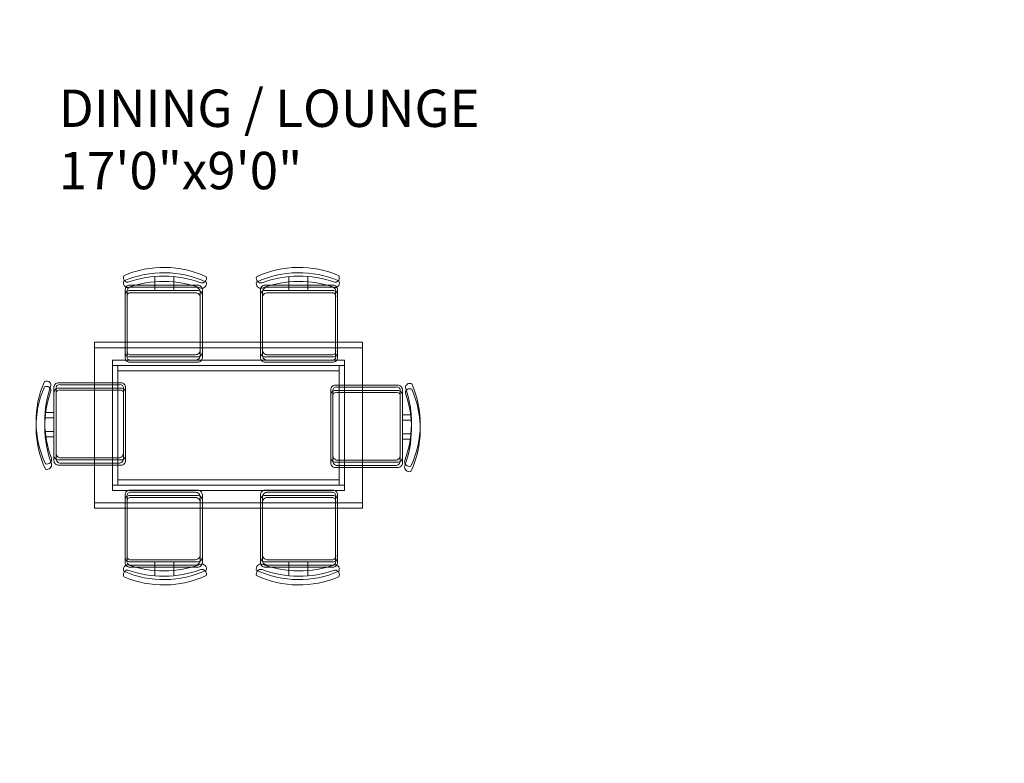
# Model space of a CAD drawing. Units: inches. Extents: x 963 to 2075, y 289 to 2657.
# Tile 14 of 98: x 1179 to 1310, y 1718 to 1818. Entities that reach past the tile are written whole.
import ezdxf

# ---------------------------------------------------------------- set-up
doc = ezdxf.new("R2010")
doc.units = ezdxf.units.IN
for name, color, linetype, lineweight in [('A-AREA-IDEN', 7, 'Continuous', 18), ('A-FURN', 8, 'Continuous', 18), ('A-WALL-PATT', 8, 'Continuous', 13)]:
    doc.layers.add(name, color=color, linetype=linetype, lineweight=lineweight)
doc.styles.get("Standard").update_dxf_attribs({"font": 'arial.ttf'})

msp = doc.modelspace()

# ---------------------------------------------------------------- hatches: boundary and pattern name
at = {"layer": 'A-WALL-PATT'}
h = msp.add_hatch(dxfattribs=at)
h.set_pattern_fill('ANSI32', color=256)
h.paths.add_polyline_path([(1296.92, 2558.32), (1203.92, 2558.32), (1203.92, 2493.82), (1191.53, 2493.82), (1191.53, 2489.32), (1211.06, 2489.32), (1211.06, 2492.02), (1211.06, 2493.82), (1208.42, 2493.82), (1208.42, 2553.82), (1292.42, 2553.82), (1292.42, 2538.86), (1296.92, 2538.86)])
h.paths.add_polyline_path([(1442.42, 2558.32), (1349.42, 2558.32), (1349.42, 2538.94), (1353.92, 2538.94), (1353.92, 2553.82), (1437.92, 2553.82), (1437.92, 2493.82), (1434.54, 2493.82), (1434.54, 2489.32), (1448.31, 2489.32), (1448.31, 2491.57), (1448.31, 2493.82), (1442.42, 2493.82)])
h.paths.add_polyline_path([(1415.55, 2491.57), (1415.55, 2493.82), (1340.94, 2493.82), (1340.94, 2489.32), (1371.92, 2489.32), (1371.92, 2378.32), (1367.6, 2378.32), (1367.6, 2373.82), (1371.92, 2373.82), (1371.92, 2355.19), (1376.42, 2355.19), (1376.42, 2489.32), (1415.55, 2489.32)])
h.paths.add_polyline_path([(1304.94, 2491.57), (1304.94, 2493.82), (1296.92, 2493.82), (1296.92, 2514.86), (1292.42, 2514.86), (1292.42, 2493.82), (1232.81, 2493.82), (1232.81, 2489.32), (1256.42, 2489.32), (1256.42, 2327.32), (1253.71, 2327.32), (1253.71, 2322.82), (1328.42, 2322.82), (1328.42, 2331.15), (1323.92, 2331.15), (1323.92, 2327.32), (1260.92, 2327.32), (1260.92, 2373.82), (1323.92, 2373.82), (1323.92, 2357.81), (1328.42, 2357.81), (1328.42, 2373.82), (1346.01, 2373.82), (1346.01, 2376.07), (1346.01, 2378.32), (1260.92, 2378.32), (1260.92, 2489.32), (1304.94, 2489.32)])
h.paths.add_polyline_path([(1226.65, 2327.32), (1124.42, 2327.32), (1124.42, 2347.45), (1119.92, 2347.45), (1119.92, 2322.82), (1163.42, 2322.82), (1163.42, 2305.43), (1165.67, 2305.43), (1167.92, 2305.43), (1167.92, 2322.82), (1226.65, 2322.82), (1226.65, 2325.07)])
h.paths.add_polyline_path([(1095.92, 2489.32), (1124.42, 2489.32), (1131.53, 2489.32), (1131.53, 2491.57), (1131.53, 2493.82), (1119.92, 2493.82), (1091.42, 2493.82), (1091.42, 2417.32), (1095.92, 2417.32), (1119.92, 2417.32), (1119.92, 2407.45), (1124.42, 2407.45), (1124.42, 2421.82), (1095.92, 2421.82)])
h.paths.add_polyline_path([(1512.92, 2558.32), (1508.42, 2558.32), (1508.42, 2493.82), (1503.4, 2493.82), (1503.4, 2489.32), (1508.42, 2489.32), (1508.42, 2327.32), (1376.42, 2327.32), (1376.42, 2330.27), (1371.92, 2330.27), (1371.92, 2298.74), (1376.42, 2298.74), (1376.42, 2322.82), (1508.42, 2322.82), (1508.42, 2165.32), (1504.26, 2165.32), (1504.26, 2160.82), (1508.42, 2160.82), (1508.42, 2108.32), (1512.92, 2108.32), (1512.92, 2160.82), (1516.18, 2160.82), (1516.18, 2163.07), (1516.18, 2165.32), (1512.92, 2165.32), (1512.92, 2322.82), (1644.92, 2322.82), (1644.92, 2298.74), (1649.42, 2298.74), (1649.42, 2322.82), (1649.42, 2330.94), (1647.17, 2330.94), (1644.92, 2330.94), (1644.92, 2327.32), (1512.92, 2327.32), (1512.92, 2489.32), (1516.76, 2489.32), (1516.76, 2491.57), (1516.76, 2493.82), (1512.92, 2493.82)])
h.paths.add_polyline_path([(1671.92, 2558.32), (1578.92, 2558.32), (1578.92, 2493.82), (1573.53, 2493.82), (1573.53, 2489.32), (1586.54, 2489.32), (1586.54, 2491.57), (1586.54, 2493.82), (1583.42, 2493.82), (1583.42, 2553.82), (1667.42, 2553.82), (1667.42, 2541.11), (1671.92, 2541.11)])
h.paths.add_polyline_path([(1681.26, 2493.82), (1671.92, 2493.82), (1671.92, 2517.11), (1667.42, 2517.11), (1667.42, 2493.82), (1610.22, 2493.82), (1610.22, 2489.32), (1644.92, 2489.32), (1644.92, 2357.87), (1649.42, 2357.87), (1649.42, 2373.82), (1652.2, 2373.82), (1652.2, 2375.83), (1652.2, 2378.32), (1649.42, 2378.32), (1649.42, 2489.32), (1681.26, 2489.32), (1681.26, 2491.57)])
h.paths.add_polyline_path([(1821.92, 2558.32), (1728.92, 2558.32), (1728.92, 2541), (1733.42, 2541), (1733.42, 2553.82), (1817.42, 2553.82), (1817.42, 2493.82), (1813.51, 2493.82), (1813.51, 2489.32), (1830.08, 2489.32), (1830.08, 2491.57), (1830.08, 2493.82), (1821.92, 2493.82)])
h.paths.add_polyline_path([(1794.24, 2493.82), (1717.26, 2493.82), (1717.26, 2489.32), (1760.42, 2489.32), (1760.42, 2378.32), (1674.4, 2378.32), (1674.4, 2373.82), (1692.92, 2373.82), (1692.92, 2356.95), (1697.42, 2356.95), (1697.42, 2373.82), (1760.42, 2373.82), (1760.42, 2327.32), (1697.42, 2327.32), (1697.42, 2333.34), (1692.92, 2333.34), (1692.92, 2322.82), (1768.04, 2322.82), (1768.04, 2325.07), (1768.04, 2327.32), (1764.92, 2327.32), (1764.92, 2489.32), (1794.24, 2489.32)])
h.paths.add_polyline_path([(1733.42, 2517), (1728.92, 2517), (1728.92, 2493.82), (1733.42, 2493.82)], flags=17)
h.paths.add_polyline_path([(1929.92, 2493.82), (1890.08, 2493.82), (1890.08, 2489.32), (1896.92, 2489.32), (1925.42, 2489.32), (1925.42, 2421.82), (1896.92, 2421.82), (1896.92, 2408.32), (1901.42, 2408.32), (1901.42, 2417.32), (1925.42, 2417.32), (1929.92, 2417.32)])
h.paths.add_polyline_path([(1901.42, 2348.32), (1896.92, 2348.32), (1896.92, 2327.32), (1800.42, 2327.32), (1800.42, 2322.82), (1853.42, 2322.82), (1853.42, 2309.45), (1857.92, 2309.45), (1857.92, 2322.82), (1901.42, 2322.82)])
h.paths.add_polyline_path([(1857.92, 2249.45), (1853.42, 2249.45), (1853.42, 2214.82), (1686.31, 2214.82), (1686.31, 2210.32), (1853.42, 2210.32), (1853.42, 2202.13), (1857.92, 2202.13), (1857.92, 2210.32)])
h.paths.add_polyline_path([(1857.92, 2142.13), (1853.42, 2142.13), (1853.42, 2115.42), (1841.42, 2115.42), (1841.42, 2088.53), (1841.42, 2046.95), (1845.92, 2046.95), (1845.92, 2110.92), (1905.92, 2110.92), (1905.92, 2092.52), (1910.42, 2092.52), (1910.42, 2115.42), (1857.92, 2115.42)])
h.paths.add_polyline_path([(1532.44, 1482.34), (1573.46, 1482.34), (1573.46, 1501), (1532.44, 1501)], flags=9)
h.paths.add_polyline_path([(1438.66, 1486.3), (1479.68, 1486.3), (1479.68, 1504.96), (1438.66, 1504.96)], flags=9)
h.paths.add_polyline_path([(1411.22, 1365.31), (1659.14, 1365.31), (1659.14, 1402.4), (1411.22, 1402.4)], flags=9)
h.paths.add_polyline_path([(1185.67, 2296.3), (1248.16, 2296.3), (1248.16, 2314.95), (1185.67, 2314.95)], flags=9)
h.paths.add_polyline_path([(1177.31, 2187.35), (1216.15, 2187.35), (1216.15, 2206.01), (1177.31, 2206.01)], flags=9)
h.paths.add_polyline_path([(1295.1, 1602.08), (1328.26, 1602.08), (1328.26, 1620.74), (1295.1, 1620.74)], flags=9)
h.paths.add_polyline_path([(1525.13, 2005.99), (1558.39, 2005.99), (1558.39, 2024.65), (1525.13, 2024.65)], flags=9)
h.paths.add_polyline_path([(1459.61, 1977.13), (1472.19, 1977.13), (1472.19, 1987.43), (1459.61, 1987.43)], flags=9)
h.paths.add_polyline_path([(1467.81, 2053.68), (1480.02, 2053.68), (1480.02, 2063.98), (1467.81, 2063.98)], flags=9)
h.paths.add_polyline_path([(1555.18, 2119.02), (1584.56, 2119.02), (1584.56, 2137.68), (1555.18, 2137.68)], flags=25)
h.paths.add_polyline_path([(1405.39, 2115.29), (1444.48, 2115.29), (1444.48, 2133.95), (1405.39, 2133.95)], flags=25)
h.paths.add_polyline_path([(1698.48, 2004.26), (1727.69, 2004.26), (1727.69, 2022.92), (1698.48, 2022.92)], flags=9)
h.paths.add_polyline_path([(1612.16, 1972.86), (1629.02, 1972.86), (1629.02, 1983.16), (1612.16, 1983.16)], flags=9)
h.paths.add_polyline_path([(1608.29, 2060.04), (1625.15, 2060.04), (1625.15, 2070.34), (1608.29, 2070.34)], flags=9)
h.paths.add_polyline_path([(1527.95, 1684.4), (1566.79, 1684.4), (1566.79, 1703.06), (1527.95, 1703.06)], flags=9)
h.paths.add_polyline_path([(1422.79, 1683.59), (1461.63, 1683.59), (1461.63, 1702.25), (1422.79, 1702.25)], flags=9)
h.paths.add_polyline_path([(1531.26, 1732.46), (1574.01, 1732.46), (1574.01, 1751.12), (1531.26, 1751.12)], flags=9)
h.paths.add_polyline_path([(1402.87, 1732.85), (1439.8, 1732.85), (1439.8, 1751.5), (1402.87, 1751.5)], flags=9)
h.paths.add_polyline_path([(1243.12, 1923.13), (1281.96, 1923.13), (1281.96, 1941.79), (1243.12, 1941.79)], flags=9)
h.paths.add_polyline_path([(1181.75, 1792.27), (1244.24, 1792.27), (1244.24, 1810.93), (1181.75, 1810.93)], flags=9)
h.paths.add_polyline_path([(1265.82, 1670.3), (1316.07, 1670.3), (1316.07, 1688.96), (1265.82, 1688.96)], flags=9)
h.paths.add_polyline_path([(1140.26, 1676.05), (1179.1, 1676.05), (1179.1, 1694.71), (1140.26, 1694.71)], flags=9)
h.paths.add_polyline_path([(1107.49, 1490.89), (1143.37, 1490.89), (1143.37, 1509.55), (1107.49, 1509.55)], flags=9)
h.paths.add_polyline_path([(1217.58, 1483.9), (1246.74, 1483.9), (1246.74, 1502.56), (1217.58, 1502.56)], flags=9)
h.paths.add_polyline_path([(1389.21, 1486.92), (1418.37, 1486.92), (1418.37, 1505.58), (1389.21, 1505.58)], flags=9)
h.paths.add_polyline_path([(1672.21, 1602.08), (1705.37, 1602.08), (1705.37, 1620.74), (1672.21, 1620.74)], flags=9)
h.paths.add_polyline_path([(1752.08, 1522.64), (1781.24, 1522.64), (1781.24, 1541.3), (1752.08, 1541.3)], flags=9)
h.paths.add_polyline_path([(1848.27, 1491.26), (1884.16, 1491.26), (1884.16, 1509.92), (1848.27, 1509.92)], flags=9)
h.paths.add_polyline_path([(1822.47, 1685.62), (1861.31, 1685.62), (1861.31, 1704.28), (1822.47, 1704.28)], flags=9)
h.paths.add_polyline_path([(1713.19, 1672.23), (1763.44, 1672.23), (1763.44, 1690.89), (1713.19, 1690.89)], flags=9)
h.paths.add_polyline_path([(1736.62, 1790.58), (1799.11, 1790.58), (1799.11, 1809.24), (1736.62, 1809.24)], flags=9)
h.paths.add_polyline_path([(1691.49, 1916.36), (1730.33, 1916.36), (1730.33, 1935.01), (1691.49, 1935.01)], flags=9)
h.paths.add_polyline_path([(1764.87, 1973.92), (1794.31, 1973.92), (1794.31, 1992.58), (1764.87, 1992.58)], flags=9)
h.paths.add_polyline_path([(1767.85, 2034.02), (1797.29, 2034.02), (1797.29, 2052.67), (1767.85, 2052.67)], flags=9)
h.paths.add_polyline_path([(1851.59, 2060.33), (1880.75, 2060.33), (1880.75, 2078.99), (1851.59, 2078.99)], flags=25)
h.paths.add_polyline_path([(1688.49, 2086.87), (1727.33, 2086.87), (1727.33, 2105.53), (1688.49, 2105.53)], flags=9)
h.paths.add_polyline_path([(1537.74, 2293.58), (1580.49, 2293.58), (1580.49, 2312.24), (1537.74, 2312.24)], flags=25)
h.paths.add_polyline_path([(1425.59, 2296.11), (1468.34, 2296.11), (1468.34, 2314.77), (1425.59, 2314.77)], flags=25)
h.paths.add_polyline_path([(1278.52, 2004.18), (1307.72, 2004.18), (1307.72, 2022.84), (1278.52, 2022.84)], flags=9)
h.paths.add_polyline_path([(1193.28, 1973.63), (1222.72, 1973.63), (1222.72, 1992.29), (1193.28, 1992.29)], flags=9)
h.paths.add_polyline_path([(1192.41, 2040.58), (1221.84, 2040.58), (1221.84, 2059.23), (1192.41, 2059.23)], flags=9)
h.paths.add_polyline_path([(1130.6, 1951.39), (1159.76, 1951.39), (1159.76, 1970.05), (1130.6, 1970.05)], flags=9)
h.paths.add_polyline_path([(1132.83, 2052.49), (1161.98, 2052.49), (1161.98, 2071.15), (1132.83, 2071.15)], flags=9)
h.paths.add_polyline_path([(1265.13, 2334.62), (1315.38, 2334.62), (1315.38, 2353.28), (1265.13, 2353.28)], flags=25)
h.paths.add_polyline_path([(1136.74, 2330.79), (1175.58, 2330.79), (1175.58, 2349.44), (1136.74, 2349.44)], flags=9)
h.paths.add_polyline_path([(1287.42, 2417.2), (1320.58, 2417.2), (1320.58, 2435.86), (1287.42, 2435.86)], flags=25)
h.paths.add_polyline_path([(1430.99, 2329.16), (1469.83, 2329.16), (1469.83, 2347.82), (1430.99, 2347.82)], flags=25)
h.paths.add_polyline_path([(1525.42, 2329.21), (1564.26, 2329.21), (1564.26, 2347.87), (1525.42, 2347.87)], flags=25)
h.paths.add_polyline_path([(1684.52, 2382.8), (1717.68, 2382.8), (1717.68, 2401.46), (1684.52, 2401.46)], flags=25)
h.paths.add_polyline_path([(1704.81, 2340.29), (1755.05, 2340.29), (1755.05, 2358.95), (1704.81, 2358.95)], flags=25)
h.paths.add_polyline_path([(1694.11, 2287.76), (1756.6, 2287.76), (1756.6, 2306.41), (1694.11, 2306.41)], flags=9)
h.paths.add_polyline_path([(1815.78, 2329.86), (1854.62, 2329.86), (1854.62, 2348.52), (1815.78, 2348.52)], flags=9)
h.paths.add_polyline_path([(1842.87, 2514.26), (1878.76, 2514.26), (1878.76, 2532.91), (1842.87, 2532.91)], flags=9)
h.paths.add_polyline_path([(1769.51, 2531.45), (1798.67, 2531.45), (1798.67, 2550.1), (1769.51, 2550.1)], flags=25)
h.paths.add_polyline_path([(1594.77, 2518.47), (1623.93, 2518.47), (1623.93, 2537.13), (1594.77, 2537.13)], flags=25)
h.paths.add_polyline_path([(1520.72, 2516.18), (1556.61, 2516.18), (1556.61, 2534.84), (1520.72, 2534.84)], flags=25)
h.paths.add_polyline_path([(1464.46, 2516.69), (1500.34, 2516.69), (1500.34, 2535.35), (1464.46, 2535.35)], flags=25)
h.paths.add_polyline_path([(1365.7, 2528.97), (1394.85, 2528.97), (1394.85, 2547.63), (1365.7, 2547.63)], flags=25)
h.paths.add_polyline_path([(1222.84, 2516.23), (1252, 2516.23), (1252, 2534.89), (1222.84, 2534.89)], flags=25)
h.paths.add_polyline_path([(1104.55, 2509.6), (1140.43, 2509.6), (1140.43, 2528.26), (1104.55, 2528.26)], flags=9)
h = msp.add_hatch(dxfattribs=at)
h.set_pattern_fill('ANSI32', color=256)
h.paths.add_polyline_path([(1335.97, 2212.57), (1335.97, 2214.82), (1167.92, 2214.82), (1167.92, 2245.43), (1163.42, 2245.43), (1163.42, 2210.32), (1163.42, 2194.81), (1167.92, 2194.81), (1167.92, 2210.32), (1335.97, 2210.32)])
h.paths.add_polyline_path([(1532.44, 1482.34), (1573.46, 1482.34), (1573.46, 1501), (1532.44, 1501)], flags=9)
h.paths.add_polyline_path([(1438.66, 1486.3), (1479.68, 1486.3), (1479.68, 1504.96), (1438.66, 1504.96)], flags=9)
h.paths.add_polyline_path([(1411.22, 1365.31), (1659.14, 1365.31), (1659.14, 1402.4), (1411.22, 1402.4)], flags=9)
h.paths.add_polyline_path([(1185.67, 2296.3), (1248.16, 2296.3), (1248.16, 2314.95), (1185.67, 2314.95)], flags=9)
h.paths.add_polyline_path([(1177.31, 2187.35), (1216.15, 2187.35), (1216.15, 2206.01), (1177.31, 2206.01)], flags=9)
h.paths.add_polyline_path([(1295.1, 1602.08), (1328.26, 1602.08), (1328.26, 1620.74), (1295.1, 1620.74)], flags=9)
h.paths.add_polyline_path([(1525.13, 2005.99), (1558.39, 2005.99), (1558.39, 2024.65), (1525.13, 2024.65)], flags=9)
h.paths.add_polyline_path([(1459.61, 1977.13), (1472.19, 1977.13), (1472.19, 1987.43), (1459.61, 1987.43)], flags=9)
h.paths.add_polyline_path([(1467.81, 2053.68), (1480.02, 2053.68), (1480.02, 2063.98), (1467.81, 2063.98)], flags=9)
h.paths.add_polyline_path([(1555.18, 2119.02), (1584.56, 2119.02), (1584.56, 2137.68), (1555.18, 2137.68)], flags=9)
h.paths.add_polyline_path([(1405.39, 2115.29), (1444.48, 2115.29), (1444.48, 2133.95), (1405.39, 2133.95)], flags=9)
h.paths.add_polyline_path([(1698.48, 2004.26), (1727.69, 2004.26), (1727.69, 2022.92), (1698.48, 2022.92)], flags=9)
h.paths.add_polyline_path([(1612.16, 1972.86), (1629.02, 1972.86), (1629.02, 1983.16), (1612.16, 1983.16)], flags=9)
h.paths.add_polyline_path([(1608.29, 2060.04), (1625.15, 2060.04), (1625.15, 2070.34), (1608.29, 2070.34)], flags=9)
h.paths.add_polyline_path([(1527.95, 1684.4), (1566.79, 1684.4), (1566.79, 1703.06), (1527.95, 1703.06)], flags=9)
h.paths.add_polyline_path([(1422.79, 1683.59), (1461.63, 1683.59), (1461.63, 1702.25), (1422.79, 1702.25)], flags=9)
h.paths.add_polyline_path([(1531.26, 1732.46), (1574.01, 1732.46), (1574.01, 1751.12), (1531.26, 1751.12)], flags=9)
h.paths.add_polyline_path([(1402.87, 1732.85), (1439.8, 1732.85), (1439.8, 1751.5), (1402.87, 1751.5)], flags=9)
h.paths.add_polyline_path([(1243.12, 1923.13), (1281.96, 1923.13), (1281.96, 1941.79), (1243.12, 1941.79)], flags=9)
h.paths.add_polyline_path([(1181.75, 1792.27), (1244.24, 1792.27), (1244.24, 1810.93), (1181.75, 1810.93)], flags=9)
h.paths.add_polyline_path([(1265.82, 1670.3), (1316.07, 1670.3), (1316.07, 1688.96), (1265.82, 1688.96)], flags=9)
h.paths.add_polyline_path([(1140.26, 1676.05), (1179.1, 1676.05), (1179.1, 1694.71), (1140.26, 1694.71)], flags=9)
h.paths.add_polyline_path([(1107.49, 1490.89), (1143.37, 1490.89), (1143.37, 1509.55), (1107.49, 1509.55)], flags=9)
h.paths.add_polyline_path([(1217.58, 1483.9), (1246.74, 1483.9), (1246.74, 1502.56), (1217.58, 1502.56)], flags=9)
h.paths.add_polyline_path([(1389.21, 1486.92), (1418.37, 1486.92), (1418.37, 1505.58), (1389.21, 1505.58)], flags=9)
h.paths.add_polyline_path([(1672.21, 1602.08), (1705.37, 1602.08), (1705.37, 1620.74), (1672.21, 1620.74)], flags=9)
h.paths.add_polyline_path([(1752.08, 1522.64), (1781.24, 1522.64), (1781.24, 1541.3), (1752.08, 1541.3)], flags=9)
h.paths.add_polyline_path([(1848.27, 1491.26), (1884.16, 1491.26), (1884.16, 1509.92), (1848.27, 1509.92)], flags=9)
h.paths.add_polyline_path([(1822.47, 1685.62), (1861.31, 1685.62), (1861.31, 1704.28), (1822.47, 1704.28)], flags=9)
h.paths.add_polyline_path([(1713.19, 1672.23), (1763.44, 1672.23), (1763.44, 1690.89), (1713.19, 1690.89)], flags=9)
h.paths.add_polyline_path([(1736.62, 1790.58), (1799.11, 1790.58), (1799.11, 1809.24), (1736.62, 1809.24)], flags=9)
h.paths.add_polyline_path([(1691.49, 1916.36), (1730.33, 1916.36), (1730.33, 1935.01), (1691.49, 1935.01)], flags=9)
h.paths.add_polyline_path([(1764.87, 1973.92), (1794.31, 1973.92), (1794.31, 1992.58), (1764.87, 1992.58)], flags=9)
h.paths.add_polyline_path([(1767.85, 2034.02), (1797.29, 2034.02), (1797.29, 2052.67), (1767.85, 2052.67)], flags=9)
h.paths.add_polyline_path([(1851.59, 2060.33), (1880.75, 2060.33), (1880.75, 2078.99), (1851.59, 2078.99)], flags=9)
h.paths.add_polyline_path([(1688.49, 2086.87), (1727.33, 2086.87), (1727.33, 2105.53), (1688.49, 2105.53)], flags=9)
h.paths.add_polyline_path([(1537.74, 2293.58), (1580.49, 2293.58), (1580.49, 2312.24), (1537.74, 2312.24)], flags=9)
h.paths.add_polyline_path([(1425.59, 2296.11), (1468.34, 2296.11), (1468.34, 2314.77), (1425.59, 2314.77)], flags=9)
h.paths.add_polyline_path([(1278.52, 2004.18), (1307.72, 2004.18), (1307.72, 2022.84), (1278.52, 2022.84)], flags=9)
h.paths.add_polyline_path([(1193.28, 1973.63), (1222.72, 1973.63), (1222.72, 1992.29), (1193.28, 1992.29)], flags=9)
h.paths.add_polyline_path([(1192.41, 2040.58), (1221.84, 2040.58), (1221.84, 2059.23), (1192.41, 2059.23)], flags=9)
h.paths.add_polyline_path([(1130.6, 1951.39), (1159.76, 1951.39), (1159.76, 1970.05), (1130.6, 1970.05)], flags=9)
h.paths.add_polyline_path([(1132.83, 2052.49), (1161.98, 2052.49), (1161.98, 2071.15), (1132.83, 2071.15)], flags=9)
h.paths.add_polyline_path([(1265.13, 2334.62), (1315.38, 2334.62), (1315.38, 2353.28), (1265.13, 2353.28)], flags=9)
h.paths.add_polyline_path([(1136.74, 2330.79), (1175.58, 2330.79), (1175.58, 2349.44), (1136.74, 2349.44)], flags=9)
h.paths.add_polyline_path([(1287.42, 2417.2), (1320.58, 2417.2), (1320.58, 2435.86), (1287.42, 2435.86)], flags=9)
h.paths.add_polyline_path([(1430.99, 2329.16), (1469.83, 2329.16), (1469.83, 2347.82), (1430.99, 2347.82)], flags=9)
h.paths.add_polyline_path([(1525.42, 2329.21), (1564.26, 2329.21), (1564.26, 2347.87), (1525.42, 2347.87)], flags=9)
h.paths.add_polyline_path([(1684.52, 2382.8), (1717.68, 2382.8), (1717.68, 2401.46), (1684.52, 2401.46)], flags=9)
h.paths.add_polyline_path([(1704.81, 2340.29), (1755.05, 2340.29), (1755.05, 2358.95), (1704.81, 2358.95)], flags=9)
h.paths.add_polyline_path([(1694.11, 2287.76), (1756.6, 2287.76), (1756.6, 2306.41), (1694.11, 2306.41)], flags=9)
h.paths.add_polyline_path([(1815.78, 2329.86), (1854.62, 2329.86), (1854.62, 2348.52), (1815.78, 2348.52)], flags=9)
h.paths.add_polyline_path([(1842.87, 2514.26), (1878.76, 2514.26), (1878.76, 2532.91), (1842.87, 2532.91)], flags=9)
h.paths.add_polyline_path([(1769.51, 2531.45), (1798.67, 2531.45), (1798.67, 2550.1), (1769.51, 2550.1)], flags=9)
h.paths.add_polyline_path([(1594.77, 2518.47), (1623.93, 2518.47), (1623.93, 2537.13), (1594.77, 2537.13)], flags=9)
h.paths.add_polyline_path([(1520.72, 2516.18), (1556.61, 2516.18), (1556.61, 2534.84), (1520.72, 2534.84)], flags=9)
h.paths.add_polyline_path([(1464.46, 2516.69), (1500.34, 2516.69), (1500.34, 2535.35), (1464.46, 2535.35)], flags=9)
h.paths.add_polyline_path([(1365.7, 2528.97), (1394.85, 2528.97), (1394.85, 2547.63), (1365.7, 2547.63)], flags=9)
h.paths.add_polyline_path([(1222.84, 2516.23), (1252, 2516.23), (1252, 2534.89), (1222.84, 2534.89)], flags=9)
h.paths.add_polyline_path([(1104.55, 2509.6), (1140.43, 2509.6), (1140.43, 2528.26), (1104.55, 2528.26)], flags=9)

# ---------------------------------------------------------------- linework, layer by layer
at = {"layer": 'A-FURN'}
for points in [[(1193, 1782.66, -0.175809), (1202.76, 1782.58, 0.578392), (1203.5, 1783.4, 0.214524), (1192.49, 1783.54, 0.552014), (1193, 1782.66, -0.065079)], [(1193, 1782.66, -0.175809), (1202.76, 1782.58, 0.578392), (1203.5, 1783.4, 0.214524), (1192.49, 1783.54, 0.552014), (1193, 1782.66, -0.065079)], [(1193, 1781.94, -0.175809), (1202.76, 1781.87, 0.578392), (1203.5, 1782.68, 0.214524), (1192.49, 1782.83, 0.552014), (1193, 1781.94, -0.065079)], [(1193, 1781.94, -0.175809), (1202.76, 1781.87, 0.578392), (1203.5, 1782.68, 0.214524), (1192.49, 1782.83, 0.552014), (1193, 1781.94, -0.065079)], [(1210.97, 1782.58, -0.578392), (1210.23, 1783.4, -0.214524), (1221.24, 1783.54, -0.552014), (1220.72, 1782.66, 0.175809), (1210.97, 1782.58)], [(1210.97, 1782.58, -0.578392), (1210.23, 1783.4, -0.214524), (1221.24, 1783.54, -0.552014), (1220.72, 1782.66, 0.175809), (1210.97, 1782.58)], [(1210.97, 1781.87, -0.578392), (1210.23, 1782.68, -0.214524), (1221.24, 1782.83, -0.552014), (1220.72, 1781.94, 0.175809), (1210.97, 1781.87)], [(1210.97, 1781.87, -0.578392), (1210.23, 1782.68, -0.214524), (1221.24, 1782.83, -0.552014), (1220.72, 1781.94, 0.175809), (1210.97, 1781.87)], [(1199.16, 1782.27), (1199.16, 1783.41, -0.064759)], [(1199.16, 1782.27), (1199.16, 1783.41, -0.064759)], [(1199.16, 1781.55), (1199.16, 1782.69, -0.064759)], [(1199.16, 1781.55), (1199.16, 1782.69, -0.064759)], [(1214.56, 1782.27), (1214.56, 1783.41, 0.064759)], [(1214.56, 1782.27), (1214.56, 1783.41, 0.064759)], [(1214.56, 1781.55), (1214.56, 1782.69, 0.064759)], [(1214.56, 1781.55), (1214.56, 1782.69, 0.064759)], [(1202.34, 1782.27), (1193.29, 1782.27, 0.414214), (1192.65, 1781.63), (1192.65, 1773.31, 0.414214), (1193.29, 1772.67), (1202.34, 1772.67, 0.414214), (1202.98, 1773.31), (1202.98, 1781.63, 0.414214), (1202.34, 1782.27)], [(1202.34, 1781.55), (1193.29, 1781.55, 0.414214), (1192.65, 1780.92), (1192.65, 1772.59, 0.414214), (1193.29, 1771.96), (1202.34, 1771.96, 0.414214), (1202.98, 1772.59), (1202.98, 1780.92, 0.414214), (1202.34, 1781.55)], [(1202.34, 1782.27), (1193.29, 1782.27, 0.414214), (1192.65, 1781.63), (1192.65, 1773.31, 0.414214), (1193.29, 1772.67), (1202.34, 1772.67, 0.414214), (1202.98, 1773.31), (1202.98, 1781.63, 0.414214), (1202.34, 1782.27)], [(1202.34, 1781.55), (1193.29, 1781.55, 0.414214), (1192.65, 1780.92), (1192.65, 1772.59, 0.414214), (1193.29, 1771.96), (1202.34, 1771.96, 0.414214), (1202.98, 1772.59), (1202.98, 1780.92, 0.414214), (1202.34, 1781.55)], [(1220.44, 1782.27, -0.414214), (1221.07, 1781.63), (1221.07, 1773.31, -0.414214), (1220.44, 1772.67), (1211.38, 1772.67, -0.414214), (1210.75, 1773.31), (1210.75, 1781.63, -0.414214), (1211.38, 1782.27), (1220.44, 1782.27)], [(1220.44, 1782.27, -0.414214), (1221.07, 1781.63), (1221.07, 1773.31, -0.414214), (1220.44, 1772.67), (1211.38, 1772.67, -0.414214), (1210.75, 1773.31), (1210.75, 1781.63, -0.414214), (1211.38, 1782.27), (1220.44, 1782.27)], [(1220.44, 1781.55, -0.414214), (1221.07, 1780.92), (1221.07, 1772.59, -0.414214), (1220.44, 1771.96), (1211.38, 1771.96, -0.414214), (1210.75, 1772.59), (1210.75, 1780.92, -0.414214), (1211.38, 1781.55), (1220.44, 1781.55)], [(1220.44, 1781.55, -0.414214), (1221.07, 1780.92), (1221.07, 1772.59, -0.414214), (1220.44, 1771.96), (1211.38, 1771.96, -0.414214), (1210.75, 1772.59), (1210.75, 1780.92, -0.414214), (1211.38, 1781.55), (1220.44, 1781.55)], [(1182.8, 1759.1, -0.578392), (1181.99, 1758.36, -0.214524), (1181.84, 1769.37, -0.552014), (1182.73, 1768.86, 0.175809), (1182.8, 1759.1)], [(1182.8, 1759.1, -0.578392), (1181.99, 1758.36, -0.214524), (1181.84, 1769.37, -0.552014), (1182.73, 1768.86, 0.175809), (1182.8, 1759.1)], [(1183.12, 1768.57, -0.414214), (1183.75, 1769.21), (1192.08, 1769.21, -0.414214), (1192.71, 1768.57), (1192.71, 1759.52, -0.414214), (1192.08, 1758.88), (1183.75, 1758.88, -0.414214), (1183.12, 1759.52), (1183.12, 1768.57)], [(1183.12, 1768.57, -0.414214), (1183.75, 1769.21), (1192.08, 1769.21, -0.414214), (1192.71, 1768.57), (1192.71, 1759.52, -0.414214), (1192.08, 1758.88), (1183.75, 1758.88, -0.414214), (1183.12, 1759.52), (1183.12, 1768.57)], [(1182.8, 1758.39, -0.578392), (1181.99, 1757.65, -0.214524), (1181.84, 1768.66, -0.552014), (1182.73, 1768.14, 0.175809), (1182.8, 1758.39)], [(1182.8, 1758.39, -0.578392), (1181.99, 1757.65, -0.214524), (1181.84, 1768.66, -0.552014), (1182.73, 1768.14, 0.175809), (1182.8, 1758.39)], [(1183.12, 1767.86, -0.414214), (1183.75, 1768.49), (1192.08, 1768.49, -0.414214), (1192.71, 1767.86), (1192.71, 1758.8, -0.414214), (1192.08, 1758.17), (1183.75, 1758.17, -0.414214), (1183.12, 1758.8), (1183.12, 1767.86)], [(1183.12, 1767.86, -0.414214), (1183.75, 1768.49), (1192.08, 1768.49, -0.414214), (1192.71, 1767.86), (1192.71, 1758.8, -0.414214), (1192.08, 1758.17), (1183.75, 1758.17, -0.414214), (1183.12, 1758.8), (1183.12, 1767.86)], [(1229.75, 1768.26, 0.414214), (1229.11, 1768.9), (1220.79, 1768.9, 0.414214), (1220.15, 1768.26), (1220.15, 1759.21, 0.414214), (1220.79, 1758.57), (1229.11, 1758.57, 0.414214), (1229.75, 1759.21), (1229.75, 1768.26)], [(1229.75, 1768.26, 0.414214), (1229.11, 1768.9), (1220.79, 1768.9, 0.414214), (1220.15, 1768.26), (1220.15, 1759.21, 0.414214), (1220.79, 1758.57), (1229.11, 1758.57, 0.414214), (1229.75, 1759.21), (1229.75, 1768.26)], [(1229.75, 1767.55, 0.414214), (1229.11, 1768.18), (1220.79, 1768.18, 0.414214), (1220.15, 1767.55), (1220.15, 1758.49, 0.414214), (1220.79, 1757.86), (1229.11, 1757.86, 0.414214), (1229.75, 1758.49), (1229.75, 1767.55)], [(1229.75, 1767.55, 0.414214), (1229.11, 1768.18), (1220.79, 1768.18, 0.414214), (1220.15, 1767.55), (1220.15, 1758.49, 0.414214), (1220.79, 1757.86), (1229.11, 1757.86, 0.414214), (1229.75, 1758.49), (1229.75, 1767.55)], [(1230.14, 1768.55, -0.175809), (1230.06, 1758.79, 0.578392), (1230.88, 1758.05, 0.214524), (1231.02, 1769.06, 0.552014), (1230.14, 1768.55, -0.065079)], [(1230.14, 1768.55, -0.175809), (1230.06, 1758.79, 0.578392), (1230.88, 1758.05, 0.214524), (1231.02, 1769.06, 0.552014), (1230.14, 1768.55, -0.065079)], [(1230.14, 1767.83, -0.175809), (1230.06, 1758.08, 0.578392), (1230.88, 1757.34, 0.214524), (1231.02, 1768.35, 0.552014), (1230.14, 1767.83, -0.065079)], [(1230.14, 1767.83, -0.175809), (1230.06, 1758.08, 0.578392), (1230.88, 1757.34, 0.214524), (1231.02, 1768.35, 0.552014), (1230.14, 1767.83, -0.065079)], [(1183.12, 1762.7), (1181.97, 1762.7, 0.064759)], [(1183.12, 1762.7), (1181.97, 1762.7, 0.064759)], [(1183.12, 1761.98), (1181.97, 1761.98, 0.064759)], [(1183.12, 1761.98), (1181.97, 1761.98, 0.064759)], [(1229.75, 1762.39), (1230.89, 1762.39, -0.064759)], [(1229.75, 1762.39), (1230.89, 1762.39, -0.064759)], [(1229.75, 1761.67), (1230.89, 1761.67, -0.064759)], [(1229.75, 1761.67), (1230.89, 1761.67, -0.064759)], [(1202.34, 1745.25), (1193.29, 1745.25, -0.414214), (1192.65, 1745.89), (1192.65, 1754.21, -0.414214), (1193.29, 1754.85), (1202.34, 1754.85, -0.414214), (1202.98, 1754.21), (1202.98, 1745.89, -0.414214), (1202.34, 1745.25)], [(1202.34, 1745.25), (1193.29, 1745.25, -0.414214), (1192.65, 1745.89), (1192.65, 1754.21, -0.414214), (1193.29, 1754.85), (1202.34, 1754.85, -0.414214), (1202.98, 1754.21), (1202.98, 1745.89, -0.414214), (1202.34, 1745.25)], [(1220.44, 1745.25, 0.414214), (1221.07, 1745.89), (1221.07, 1754.21, 0.414214), (1220.44, 1754.85), (1211.38, 1754.85, 0.414214), (1210.75, 1754.21), (1210.75, 1745.89, 0.414214), (1211.38, 1745.25), (1220.44, 1745.25)], [(1220.44, 1745.25, 0.414214), (1221.07, 1745.89), (1221.07, 1754.21, 0.414214), (1220.44, 1754.85), (1211.38, 1754.85, 0.414214), (1210.75, 1754.21), (1210.75, 1745.89, 0.414214), (1211.38, 1745.25), (1220.44, 1745.25)], [(1202.34, 1744.54), (1193.29, 1744.54, -0.414214), (1192.65, 1745.17), (1192.65, 1753.5, -0.414214), (1193.29, 1754.13), (1202.34, 1754.13, -0.414214), (1202.98, 1753.5), (1202.98, 1745.17, -0.414214), (1202.34, 1744.54)], [(1202.34, 1744.54), (1193.29, 1744.54, -0.414214), (1192.65, 1745.17), (1192.65, 1753.5, -0.414214), (1193.29, 1754.13), (1202.34, 1754.13, -0.414214), (1202.98, 1753.5), (1202.98, 1745.17, -0.414214), (1202.34, 1744.54)], [(1220.44, 1744.54, 0.414214), (1221.07, 1745.17), (1221.07, 1753.5, 0.414214), (1220.44, 1754.13), (1211.38, 1754.13, 0.414214), (1210.75, 1753.5), (1210.75, 1745.17, 0.414214), (1211.38, 1744.54), (1220.44, 1744.54)], [(1220.44, 1744.54, 0.414214), (1221.07, 1745.17), (1221.07, 1753.5, 0.414214), (1220.44, 1754.13), (1211.38, 1754.13, 0.414214), (1210.75, 1753.5), (1210.75, 1745.17, 0.414214), (1211.38, 1744.54), (1220.44, 1744.54)], [(1202.76, 1744.94, -0.578392), (1203.5, 1744.12, -0.214524), (1192.49, 1743.98, -0.552014), (1193, 1744.86, 0.175809), (1202.76, 1744.94)], [(1202.76, 1744.94, -0.578392), (1203.5, 1744.12, -0.214524), (1192.49, 1743.98, -0.552014), (1193, 1744.86, 0.175809), (1202.76, 1744.94)], [(1202.76, 1744.22, -0.578392), (1203.5, 1743.41, -0.214524), (1192.49, 1743.26, -0.552014), (1193, 1744.15, 0.175809), (1202.76, 1744.22)], [(1202.76, 1744.22, -0.578392), (1203.5, 1743.41, -0.214524), (1192.49, 1743.26, -0.552014), (1193, 1744.15, 0.175809), (1202.76, 1744.22)], [(1199.16, 1745.25), (1199.16, 1744.11, 0.064759)], [(1199.16, 1745.25), (1199.16, 1744.11, 0.064759)], [(1199.16, 1744.54), (1199.16, 1743.39, 0.064759)], [(1199.16, 1744.54), (1199.16, 1743.39, 0.064759)], [(1220.72, 1744.86, -0.175809), (1210.97, 1744.94, 0.578392), (1210.23, 1744.12, 0.214524), (1221.24, 1743.98, 0.552014), (1220.72, 1744.86, -0.065079)], [(1220.72, 1744.86, -0.175809), (1210.97, 1744.94, 0.578392), (1210.23, 1744.12, 0.214524), (1221.24, 1743.98, 0.552014), (1220.72, 1744.86, -0.065079)], [(1220.72, 1744.15, -0.175809), (1210.97, 1744.22, 0.578392), (1210.23, 1743.41, 0.214524), (1221.24, 1743.26, 0.552014), (1220.72, 1744.15, -0.065079)], [(1220.72, 1744.15, -0.175809), (1210.97, 1744.22, 0.578392), (1210.23, 1743.41, 0.214524), (1221.24, 1743.26, 0.552014), (1220.72, 1744.15, -0.065079)], [(1214.56, 1745.25), (1214.56, 1744.11, -0.064759)], [(1214.56, 1745.25), (1214.56, 1744.11, -0.064759)], [(1214.56, 1744.54), (1214.56, 1743.39, -0.064759)], [(1214.56, 1744.54), (1214.56, 1743.39, -0.064759)]]:
    msp.add_lwpolyline(points, format="xyb", dxfattribs=at)
for points in [[(1196.63, 1783.43), (1196.63, 1782.27)], [(1196.63, 1783.43), (1196.63, 1782.27)], [(1196.63, 1782.72), (1196.63, 1781.55)], [(1196.63, 1782.72), (1196.63, 1781.55)], [(1217.1, 1783.43), (1217.1, 1782.27)], [(1217.1, 1783.43), (1217.1, 1782.27)], [(1217.1, 1782.72), (1217.1, 1781.55)], [(1217.1, 1782.72), (1217.1, 1781.55)], [(1181.95, 1765.23), (1183.12, 1765.23)], [(1181.95, 1765.23), (1183.12, 1765.23)], [(1181.95, 1764.52), (1183.12, 1764.52)], [(1181.95, 1764.52), (1183.12, 1764.52)], [(1230.91, 1764.92), (1229.75, 1764.92)], [(1230.91, 1764.92), (1229.75, 1764.92)], [(1230.91, 1764.21), (1229.75, 1764.21)], [(1230.91, 1764.21), (1229.75, 1764.21)], [(1196.63, 1744.09), (1196.63, 1745.25)], [(1196.63, 1744.09), (1196.63, 1745.25)], [(1196.63, 1743.37), (1196.63, 1744.54)], [(1196.63, 1743.37), (1196.63, 1744.54)], [(1217.1, 1744.09), (1217.1, 1745.25)], [(1217.1, 1744.09), (1217.1, 1745.25)], [(1217.1, 1743.37), (1217.1, 1744.54)], [(1217.1, 1743.37), (1217.1, 1744.54)]]:
    msp.add_lwpolyline(points, dxfattribs=at)
for points in [[(1193.29, 1781.98), (1202.06, 1781.98, -0.414214), (1202.69, 1781.35), (1202.69, 1773.59, -0.414214), (1202.06, 1772.96), (1193.29, 1772.96, -0.512069), (1192.94, 1773.59), (1192.94, 1781.35, -0.512069)], [(1193.29, 1781.98), (1202.06, 1781.98, -0.414214), (1202.69, 1781.35), (1202.69, 1773.59, -0.414214), (1202.06, 1772.96), (1193.29, 1772.96, -0.512069), (1192.94, 1773.59), (1192.94, 1781.35, -0.512069)], [(1193.29, 1781.26), (1202.06, 1781.26, -0.414214), (1202.69, 1780.63), (1202.69, 1772.88, -0.414214), (1202.06, 1772.24), (1193.29, 1772.24, -0.512069), (1192.94, 1772.88), (1192.94, 1780.63, -0.512069)], [(1193.29, 1781.26), (1202.06, 1781.26, -0.414214), (1202.69, 1780.63), (1202.69, 1772.88, -0.414214), (1202.06, 1772.24), (1193.29, 1772.24, -0.512069), (1192.94, 1772.88), (1192.94, 1780.63, -0.512069)], [(1220.43, 1781.98), (1211.67, 1781.98, 0.414214), (1211.03, 1781.35), (1211.03, 1773.59, 0.414214), (1211.67, 1772.96), (1220.43, 1772.96, 0.512069), (1220.79, 1773.59), (1220.79, 1781.35, 0.512069)], [(1220.43, 1781.98), (1211.67, 1781.98, 0.414214), (1211.03, 1781.35), (1211.03, 1773.59, 0.414214), (1211.67, 1772.96), (1220.43, 1772.96, 0.512069), (1220.79, 1773.59), (1220.79, 1781.35, 0.512069)], [(1220.43, 1781.26), (1211.67, 1781.26, 0.414214), (1211.03, 1780.63), (1211.03, 1772.88, 0.414214), (1211.67, 1772.24), (1220.43, 1772.24, 0.512069), (1220.79, 1772.88), (1220.79, 1780.63, 0.512069)], [(1220.43, 1781.26), (1211.67, 1781.26, 0.414214), (1211.03, 1780.63), (1211.03, 1772.88, 0.414214), (1211.67, 1772.24), (1220.43, 1772.24, 0.512069), (1220.79, 1772.88), (1220.79, 1780.63, 0.512069)], [(1183.4, 1768.57), (1183.4, 1759.8, 0.414214), (1184.04, 1759.17), (1191.79, 1759.17, 0.414214), (1192.42, 1759.8), (1192.42, 1768.57, 0.512069), (1191.79, 1768.92), (1184.04, 1768.92, 0.512069)], [(1183.4, 1768.57), (1183.4, 1759.8, 0.414214), (1184.04, 1759.17), (1191.79, 1759.17, 0.414214), (1192.42, 1759.8), (1192.42, 1768.57, 0.512069), (1191.79, 1768.92), (1184.04, 1768.92, 0.512069)], [(1183.4, 1767.85), (1183.4, 1759.09, 0.414214), (1184.04, 1758.45), (1191.79, 1758.45, 0.414214), (1192.42, 1759.09), (1192.42, 1767.85, 0.512069), (1191.79, 1768.2), (1184.04, 1768.2, 0.512069)], [(1183.4, 1767.85), (1183.4, 1759.09, 0.414214), (1184.04, 1758.45), (1191.79, 1758.45, 0.414214), (1192.42, 1759.09), (1192.42, 1767.85, 0.512069), (1191.79, 1768.2), (1184.04, 1768.2, 0.512069)], [(1229.46, 1768.26), (1229.46, 1759.49, -0.414214), (1228.83, 1758.86), (1221.07, 1758.86, -0.414214), (1220.44, 1759.49), (1220.44, 1768.26, -0.512069), (1221.07, 1768.61), (1228.83, 1768.61, -0.512069)], [(1229.46, 1768.26), (1229.46, 1759.49, -0.414214), (1228.83, 1758.86), (1221.07, 1758.86, -0.414214), (1220.44, 1759.49), (1220.44, 1768.26, -0.512069), (1221.07, 1768.61), (1228.83, 1768.61, -0.512069)], [(1229.46, 1767.54), (1229.46, 1758.78, -0.414214), (1228.83, 1758.14), (1221.07, 1758.14, -0.414214), (1220.44, 1758.78), (1220.44, 1767.54, -0.512069), (1221.07, 1767.89), (1228.83, 1767.89, -0.512069)], [(1229.46, 1767.54), (1229.46, 1758.78, -0.414214), (1228.83, 1758.14), (1221.07, 1758.14, -0.414214), (1220.44, 1758.78), (1220.44, 1767.54, -0.512069), (1221.07, 1767.89), (1228.83, 1767.89, -0.512069)], [(1193.29, 1745.54), (1202.06, 1745.54, 0.414214), (1202.69, 1746.17), (1202.69, 1753.93, 0.414214), (1202.06, 1754.56), (1193.29, 1754.56, 0.512069), (1192.94, 1753.93), (1192.94, 1746.17, 0.512069)], [(1193.29, 1745.54), (1202.06, 1745.54, 0.414214), (1202.69, 1746.17), (1202.69, 1753.93, 0.414214), (1202.06, 1754.56), (1193.29, 1754.56, 0.512069), (1192.94, 1753.93), (1192.94, 1746.17, 0.512069)], [(1193.29, 1744.82), (1202.06, 1744.82, 0.414214), (1202.69, 1745.46), (1202.69, 1753.21, 0.414214), (1202.06, 1753.85), (1193.29, 1753.85, 0.512069), (1192.94, 1753.21), (1192.94, 1745.46, 0.512069)], [(1193.29, 1744.82), (1202.06, 1744.82, 0.414214), (1202.69, 1745.46), (1202.69, 1753.21, 0.414214), (1202.06, 1753.85), (1193.29, 1753.85, 0.512069), (1192.94, 1753.21), (1192.94, 1745.46, 0.512069)], [(1220.43, 1745.54), (1211.67, 1745.54, -0.414214), (1211.03, 1746.17), (1211.03, 1753.93, -0.414214), (1211.67, 1754.56), (1220.43, 1754.56, -0.512069), (1220.79, 1753.93), (1220.79, 1746.17, -0.512069)], [(1220.43, 1745.54), (1211.67, 1745.54, -0.414214), (1211.03, 1746.17), (1211.03, 1753.93, -0.414214), (1211.67, 1754.56), (1220.43, 1754.56, -0.512069), (1220.79, 1753.93), (1220.79, 1746.17, -0.512069)], [(1220.43, 1744.82), (1211.67, 1744.82, -0.414214), (1211.03, 1745.46), (1211.03, 1753.21, -0.414214), (1211.67, 1753.85), (1220.43, 1753.85, -0.512069), (1220.79, 1753.21), (1220.79, 1745.46, -0.512069)], [(1220.43, 1744.82), (1211.67, 1744.82, -0.414214), (1211.03, 1745.46), (1211.03, 1753.21, -0.414214), (1211.67, 1753.85), (1220.43, 1753.85, -0.512069), (1220.79, 1753.21), (1220.79, 1745.46, -0.512069)]]:
    msp.add_lwpolyline(points, format="xyb", close=True, dxfattribs=at)
for points in [[(1188.57, 1774.62), (1224.39, 1774.62), (1224.39, 1753.13), (1188.57, 1753.13)], [(1188.57, 1774.62), (1224.39, 1774.62), (1224.39, 1753.13), (1188.57, 1753.13)], [(1188.57, 1773.9), (1224.39, 1773.9), (1224.39, 1752.42), (1188.57, 1752.42)], [(1188.57, 1773.9), (1224.39, 1773.9), (1224.39, 1752.42), (1188.57, 1752.42)], [(1190.96, 1772.23), (1222, 1772.23), (1222, 1755.52), (1190.96, 1755.52)], [(1190.96, 1772.23), (1222, 1772.23), (1222, 1755.52), (1190.96, 1755.52)], [(1190.96, 1771.51), (1222, 1771.51), (1222, 1754.8), (1190.96, 1754.8)], [(1190.96, 1771.51), (1222, 1771.51), (1222, 1754.8), (1190.96, 1754.8)], [(1191.68, 1771.51), (1221.28, 1771.51), (1221.28, 1756.24), (1191.68, 1756.24)], [(1191.68, 1771.51), (1221.28, 1771.51), (1221.28, 1756.24), (1191.68, 1756.24)], [(1191.68, 1770.8), (1221.28, 1770.8), (1221.28, 1755.52), (1191.68, 1755.52)], [(1191.68, 1770.8), (1221.28, 1770.8), (1221.28, 1755.52), (1191.68, 1755.52)]]:
    msp.add_lwpolyline(points, close=True, dxfattribs=at)

# ---------------------------------------------------------------- texts
at = {"layer": 'A-AREA-IDEN', "insert": (1183.76, 1808.44), "char_height": 5, "attachment_point": 1}
msp.add_mtext_dynamic_manual_height_columns('DINING / LOUNGE\\P17\'0"x9\'0"', width=188.1595, gutter_width=12.5, heights=[0], dxfattribs=at)

doc.saveas('drawing.dxf')
